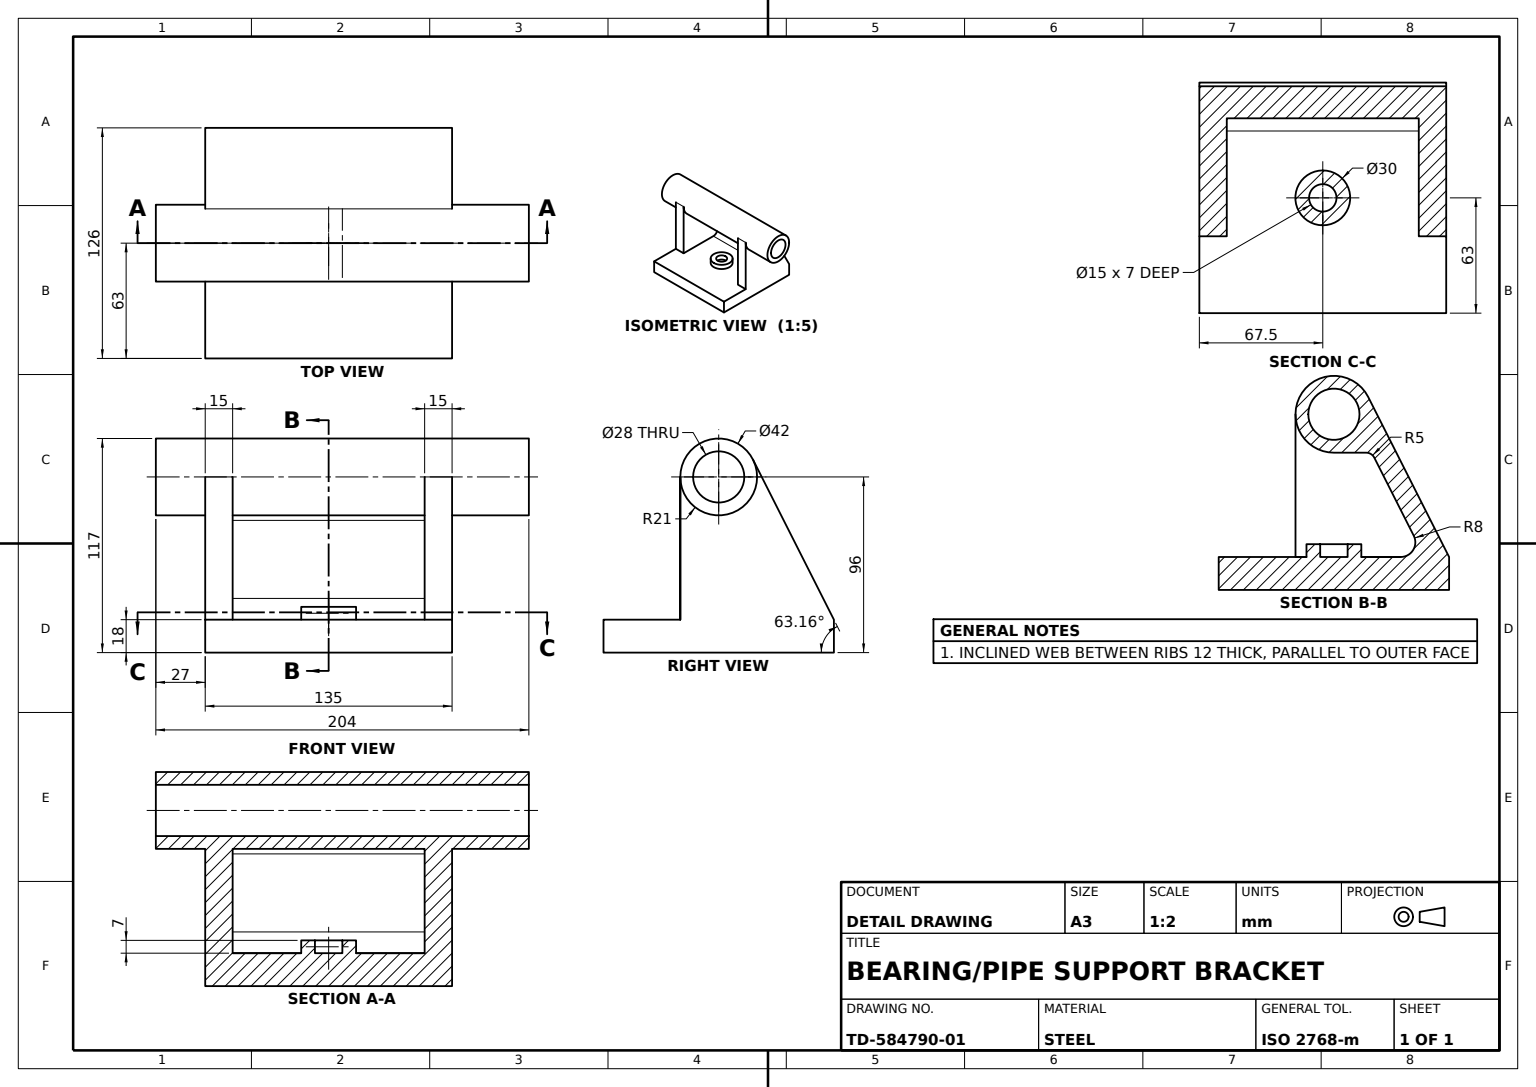
SolidWorks part; units mm, degrees
material "Plain Carbon Steel"
ref_plane "Front Plane" through (0, 0, 0) normal (0, 0, 1) x (1, 0, 0)
ref_plane "Top Plane" through (0, 0, 0) normal (0, 1, 0) x (1, 0, 0)
ref_plane "Right Plane" through (0, 0, 0) normal (1, 0, 0) x (0, 0, -1)
sketch "Pedestal Section Sketch" plane through (0, 0, 0) normal (1, 0, 0) x (0, 0, -1)
  line L0 (0, 0) -> (63, 0)
  line L1 (63, 0) -> (63, 18)
  line L2 (0, 0) -> (0, 96) construction
  line L3 (63, 18) -> (18.7381, 105.4808)
  line L4 (0, 0) -> (-63, 0)
  line L5 (-63, 0) -> (-63, 18)
  line L8 (-21, 96) -> (-21, 18)
  line L9 (43.6764, 29.6117) -> (22.0993, 72.2573)
  line L10 (0, 75) -> (17.6379, 75)
  line L11 (-63, 18) -> (63, 18)
  circle A1 centre (0, 96) radius 21
  circle A3 centre (0, 96) radius 14
  arc A7 (22.0993, 72.2573) -> (17.6379, 75) centre (17.6379, 70) ccw
  arc A8 (36.538, 18) -> (43.6764, 29.6117) centre (36.538, 26) ccw
  dimension "D1" = 12
  dimension "D4" = 42
  dimension "D5" = 28
  dimension "D6" = 8
  dimension "D9" = 5
  dimension "D2" = 63
  dimension "D3" = 63
  dimension "D7" = 18
  dimension "D8" = 18
  dimension "D10" = 96
extrude "Pedestal Body 135mm" add sketch "Pedestal Section Sketch" along normal mid plane 135
sketch "Tube Extension Short Sketch Ø42xØ28" plane through (-67.5, 0, 0) normal (-1, 0, 0) x (0, 0, 1)
  circle A0 centre (0, 96) radius 14
  circle A1 centre (0, 96) radius 21
  dimension "D1" = 42
  dimension "D2" = 28
extrude "Tube Extension 27mm" add sketch "Tube Extension Short Sketch Ø42xØ28" along normal blind 27
sketch "Tube Extension Long Sketch Ø42xØ28" plane through (67.5, 0, 0) normal (1, 0, 0) x (0, 0, -1)
  circle A0 centre (0, 96) radius 14
  circle A1 centre (0, 96) radius 21
  dimension "D1" = 42
  dimension "D2" = 28
extrude "Tube Extension 42mm" add sketch "Tube Extension Long Sketch Ø42xØ28" along normal blind 42
sketch "Support Rib A Sketch" plane through (67.5, 0, 0) normal (1, 0, 0) x (0, 0, -1)
  line L0 (-21, 96) -> (-21, 18)
  line L1 (-63, 18) -> (36.538, 18) construction
  line L2 (-21, 18) -> (36.538, 18)
  line L3 (43.6764, 29.6117) -> (22.0993, 72.2573)
  line L4 (17.6379, 75) -> (0, 75)
  circle A0 centre (0, 96) radius 21 construction
  arc A1 (36.538, 18) -> (43.6764, 29.6117) centre (36.538, 26) ccw
  arc A2 (36.538, 18) -> (43.6764, 29.6117) centre (36.538, 26) ccw construction
  arc A3 (22.0993, 72.2573) -> (17.6379, 75) centre (17.6379, 70) ccw
  arc A4 (0, 75) -> (-21, 96) centre (0, 96) cw
extrude "Support Rib A" add sketch "Support Rib A Sketch" against normal blind 15
sketch "Support Rib B Sketch" plane through (-67.5, 0, 0) normal (-1, 0, 0) x (0, 0, 1)
  line L0 (21, 96) -> (21, 18)
  line L1 (21, 18) -> (-36.538, 18)
  line L2 (-43.6764, 29.6117) -> (-22.0993, 72.2573)
  line L3 (-17.6379, 75) -> (0, 75)
  arc A0 (-43.6764, 29.6117) -> (-36.538, 18) centre (-36.538, 26) ccw construction
  arc A1 (-43.6764, 29.6117) -> (-36.538, 18) centre (-36.538, 26) ccw construction
  arc A2 (-36.538, 18) -> (-43.6764, 29.6117) centre (-36.538, 26) cw
  arc A3 (-22.0993, 72.2573) -> (-17.6379, 75) centre (-17.6379, 70) cw
  circle A4 centre (0, 96) radius 21 construction
  arc A5 (0, 75) -> (21, 96) centre (0, 96) ccw construction
  arc A6 (0, 75) -> (21, 96) centre (0, 96) ccw
  dimension "D1" = 5
extrude "Support Rib B" add sketch "Support Rib B Sketch" against normal blind 15
sketch "Base Boss Sketch Ø30xØ15" plane through (0, 18, 0) normal (0, 1, 0) x (1, 0, 0)
  circle A0 centre (0, 0) radius 15
  circle A1 centre (0, 0) radius 7.5
  dimension "D1" = 30
  dimension "D2" = 15
extrude "Base Boss Ø30xØ15" add sketch "Base Boss Sketch Ø30xØ15" along normal blind 7
